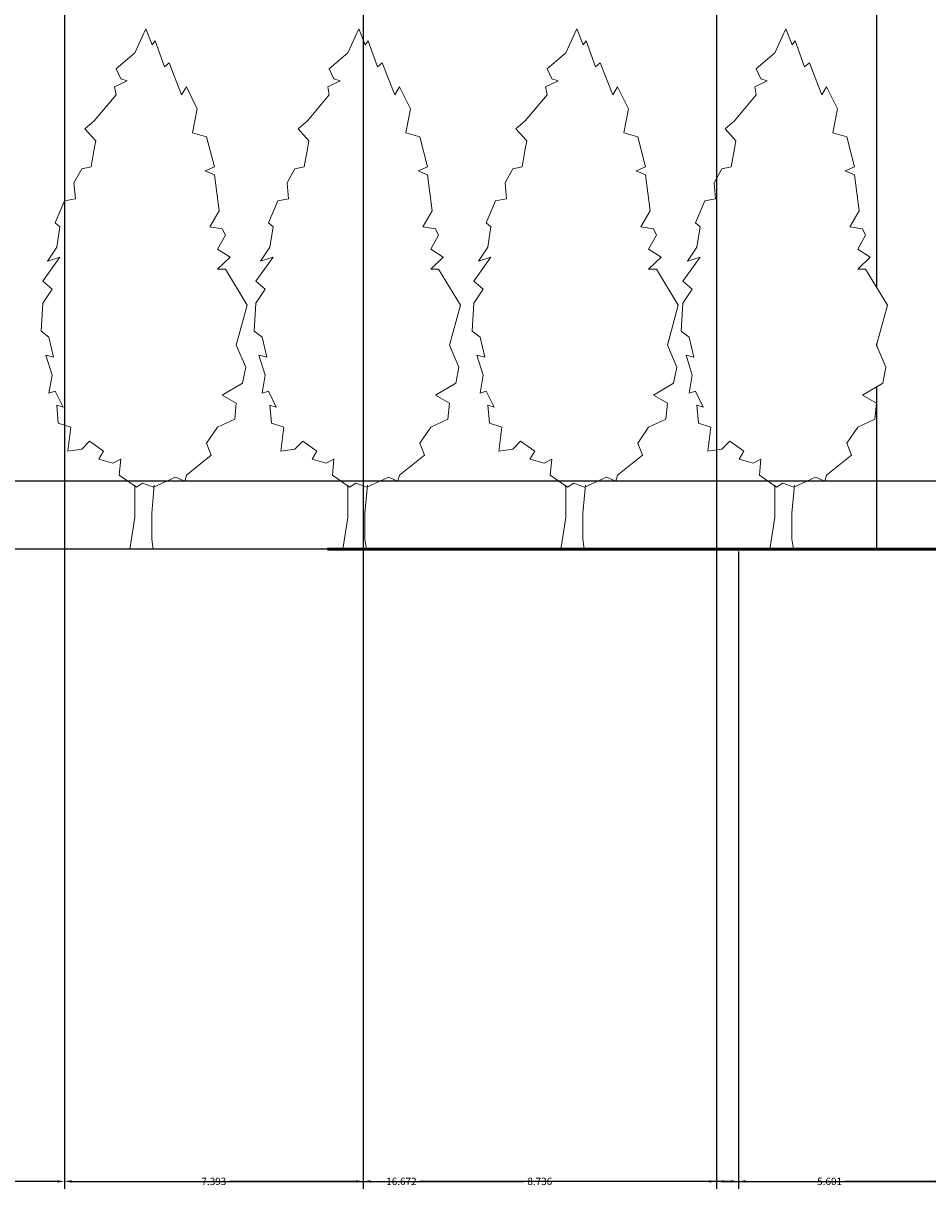
# Model space of a CAD drawing. Units: inches. Extents: x -117 to 121, y -77 to 40.
# Tile 2 of 45: x -95 to -73, y -77 to -48. Entities that reach past the tile are written whole.
import ezdxf

# ---------------------------------------------------------------- set-up
doc = ezdxf.new("R2010")
doc.units = ezdxf.units.IN
doc.header["$MEASUREMENT"] = 0
for name, color, linetype, lineweight in [('A-ANNO-DIMS', 2, 'Continuous', 18), ('A-ELEV', 7, 'Continuous', 25), ('A-ELEV-GRND', 7, 'Continuous', 50), ('L-PLNT', 3, 'Continuous', 13)]:
    doc.layers.add(name, color=color, linetype=linetype, lineweight=lineweight)
doc.styles.get("Standard").update_dxf_attribs({"font": 'arial.ttf'})
doc.dimstyles.get("Standard").update_dxf_attribs({"dimtxt": 0.18, "dimasz": 0.18, "dimexe": 0.18, "dimexo": 0.0625, "dimgap": 0.09, "dimtad": 0, "dimtih": 1, "dimtoh": 1, "dimdec": 4, "dimzin": 0, "dimdsep": 46, "dimtxsty": 'Standard', "dimcen": 0.09, "dimadec": 0, "dimazin": 0, "dimtfac": 1, "dimtdec": 4, "dimtofl": 0, "dimtmove": 0, "dimatfit": 3, "dimfxl": 1, "dimtolj": 1, "dimtzin": 0, "dimarcsym": 0})

# ---------------------------------------------------------------- blocks, each defined once
blk = doc.blocks.new('*U2')
blk.add_lwpolyline([(-2.754, 191.699), (-6.78, 182.851), (-13.682, 176.953), (-11.956, 173.266), (-9.656, 172.529), (-14.257, 170.317), (-13.682, 167.368), (-21.733, 157.783), (-25.184, 154.834), (-21.158, 150.41), (-21.733, 147.461), (-22.884, 140.825), (-26.334, 140.087), (-29.21, 134.926), (-28.635, 129.028), (-32.661, 128.291), (-36.111, 120.18), (-34.386, 118.706), (-35.536, 111.333), (-38.987, 106.171), (-34.386, 107.646), (-40.712, 98.798), (-37.261, 95.849), (-40.712, 90.688), (-41.287, 80.366), (-38.412, 78.154), (-36.686, 70.781), (-39.562, 71.518), (-37.261, 64.145), (-38.412, 57.509), (-36.111, 58.247), (-33.236, 52.348), (-35.536, 53.086), (-34.961, 46.45), (-30.36, 44.975), (-31.51, 36.128), (-26.334, 36.865), (-23.459, 39.814), (-18.283, 36.128), (-20.008, 33.178), (-14.832, 31.704), (-11.956, 33.178), (-12.531, 27.28), (-6.205, 22.856), (-3.905, 24.331), (0.121, 22.856), (8.173, 26.543), (11.624, 25.068), (12.199, 27.28), (21.4, 34.653), (19.675, 39.077), (23.701, 44.975), (30.027, 47.924), (30.602, 53.823), (25.426, 56.772), (32.903, 61.196), (34.053, 67.094), (30.602, 75.205), (34.628, 89.951), (26.576, 103.222), (23.701, 103.222), (28.302, 107.646), (23.701, 110.595), (26.576, 115.756), (25.426, 117.968), (20.825, 118.706), (24.276, 124.604), (22.551, 137.876), (19.1, 139.35), (22.551, 140.825), (19.675, 151.884), (14.499, 153.359), (16.224, 162.207), (12.199, 170.317), (10.473, 167.368), (5.872, 179.165), (4.147, 177.69), (0.696, 187.275), (-0.454, 185.8)], close=True)
for points in [[(-6.813, 23.669), (-6.813, 11.669), (-8.627, 0)], [(0.387, 23.669), (-0.576, 13.271), (-0.576, 3.686), (0, 0)]]:
    blk.add_lwpolyline(points)
blk = doc.blocks.new('*D5')
at = {"layer": 'A-ANNO-DIMS', "color": 0, "lineweight": -2, "transparency": 16777216}
for p, q in [((-94.436, -23.563), (-94.436, -77.193)), ((-106.034, -61.438), (-106.034, -77.193)), ((-105.854, -77.013), (-100.69, -77.013)), ((-94.616, -77.013), (-99.779, -77.013))]:
    blk.add_line(p, q, dxfattribs=at)
at = {"layer": 'A-ANNO-DIMS', "color": 0, "transparency": 16777216}
for points in [[(-105.854, -76.983), (-105.854, -77.043), (-106.034, -77.013)], [(-94.616, -76.983), (-94.616, -77.043), (-94.436, -77.013)]]:
    blk.add_solid(points, dxfattribs=at)
at = {"layer": 'Defpoints', "color": 0, "transparency": 16777216}
for p in [(-94.436, -23.501), (-106.034, -61.376), (-94.436, -77.013)]:
    blk.add_point(p, dxfattribs=at)
at = {"layer": 'A-ANNO-DIMS', "color": 0, "transparency": 16777216, "insert": (-100.235, -77.013), "char_height": 0.18, "attachment_point": 5}
blk.add_mtext('\\A1;11.598', dxfattribs=at)
blk = doc.blocks.new('*D6')
at = {"layer": 'A-ANNO-DIMS', "color": 0, "lineweight": -2, "transparency": 16777216}
for p, q in [((-94.436, -23.563), (-94.436, -77.193)), ((-77.763, -61.431), (-77.763, -77.193)), ((-94.256, -77.013), (-86.554, -77.013)), ((-77.943, -77.013), (-85.645, -77.013))]:
    blk.add_line(p, q, dxfattribs=at)
at = {"layer": 'A-ANNO-DIMS', "color": 0, "transparency": 16777216}
for points in [[(-94.256, -76.983), (-94.256, -77.043), (-94.436, -77.013)], [(-77.943, -76.983), (-77.943, -77.043), (-77.763, -77.013)]]:
    blk.add_solid(points, dxfattribs=at)
at = {"layer": 'Defpoints', "color": 0, "transparency": 16777216}
for p in [(-94.436, -23.501), (-77.763, -61.369), (-77.763, -77.013)]:
    blk.add_point(p, dxfattribs=at)
at = {"layer": 'A-ANNO-DIMS', "color": 0, "transparency": 16777216, "insert": (-86.099, -77.013), "char_height": 0.18, "attachment_point": 5}
blk.add_mtext('\\A1;16.672', dxfattribs=at)
blk = doc.blocks.new('*D7')
at = {"layer": 'A-ANNO-DIMS', "color": 0, "lineweight": -2, "transparency": 16777216}
for p, q in [((-77.763, -61.431), (-77.763, -77.193)), ((90.549, -61.438), (90.549, -77.193)), ((-77.583, -77.013), (6.008, -77.013)), ((90.369, -77.013), (6.778, -77.013))]:
    blk.add_line(p, q, dxfattribs=at)
at = {"layer": 'A-ANNO-DIMS', "color": 0, "transparency": 16777216}
for points in [[(-77.583, -76.983), (-77.583, -77.043), (-77.763, -77.013)], [(90.369, -76.983), (90.369, -77.043), (90.549, -77.013)]]:
    blk.add_solid(points, dxfattribs=at)
at = {"layer": 'Defpoints', "color": 0, "transparency": 16777216}
for p in [(-77.763, -61.369), (90.549, -61.376), (90.549, -77.013)]:
    blk.add_point(p, dxfattribs=at)
at = {"layer": 'A-ANNO-DIMS', "color": 0, "transparency": 16777216, "insert": (6.393, -77.013), "char_height": 0.18, "attachment_point": 5}
blk.add_mtext('\\A1;168.3', dxfattribs=at)
blk = doc.blocks.new('*D13')
at = {"layer": 'A-ANNO-DIMS', "color": 0, "lineweight": -2, "transparency": 16777216}
for p, q in [((-2.663, 27.063), (-117.024, 27.063)), ((-116.844, 26.883), (-116.844, -16.974)), ((-116.844, -61.196), (-116.844, -17.338)), ((-106.096, -61.376), (-117.024, -61.376))]:
    blk.add_line(p, q, dxfattribs=at)
at = {"layer": 'A-ANNO-DIMS', "color": 0, "transparency": 16777216}
for points in [[(-116.874, 26.883), (-116.814, 26.883), (-116.844, 27.063)], [(-116.874, -61.196), (-116.814, -61.196), (-116.844, -61.376)]]:
    blk.add_solid(points, dxfattribs=at)
at = {"layer": 'Defpoints', "color": 0, "transparency": 16777216}
for p in [(-2.6, 27.063), (-116.844, -61.376), (-106.034, -61.376)]:
    blk.add_point(p, dxfattribs=at)
at = {"layer": 'A-ANNO-DIMS', "color": 0, "transparency": 16777216, "insert": (-116.844, -17.156), "char_height": 0.18, "attachment_point": 5}
blk.add_mtext('\\A1;88.44', dxfattribs=at)
blk = doc.blocks.new('*D18')
at = {"layer": 'A-ANNO-DIMS', "color": 0, "lineweight": -2, "transparency": 16777216}
for p, q in [((-94.498, -23.501), (-117.024, -23.501)), ((-116.844, -23.681), (-116.844, -42.253)), ((-116.844, -61.189), (-116.844, -42.617)), ((-77.826, -61.369), (-117.024, -61.369))]:
    blk.add_line(p, q, dxfattribs=at)
at = {"layer": 'A-ANNO-DIMS', "color": 0, "transparency": 16777216}
for points in [[(-116.874, -23.681), (-116.814, -23.681), (-116.844, -23.501)], [(-116.874, -61.189), (-116.814, -61.189), (-116.844, -61.369)]]:
    blk.add_solid(points, dxfattribs=at)
at = {"layer": 'Defpoints', "color": 0, "transparency": 16777216}
for p in [(-94.436, -23.501), (-116.844, -61.369), (-77.763, -61.369)]:
    blk.add_point(p, dxfattribs=at)
at = {"layer": 'A-ANNO-DIMS', "color": 0, "transparency": 16777216, "insert": (-116.844, -42.435), "char_height": 0.18, "attachment_point": 5}
blk.add_mtext('\\A1;37.87', dxfattribs=at)
blk = doc.blocks.new('*D21')
at = {"layer": 'A-ANNO-DIMS', "color": 0, "lineweight": -2, "transparency": 16777216}
for p, q in [((-106.034, -61.313), (-106.034, 38.61)), ((-105.854, 38.43), (-91.382, 38.43)), ((-75.984, 38.43), (-90.455, 38.43)), ((-75.804, 8.087), (-75.804, 38.61))]:
    blk.add_line(p, q, dxfattribs=at)
at = {"layer": 'A-ANNO-DIMS', "color": 0, "transparency": 16777216}
for points in [[(-105.854, 38.46), (-105.854, 38.4), (-106.034, 38.43)], [(-75.984, 38.46), (-75.984, 38.4), (-75.804, 38.43)]]:
    blk.add_solid(points, dxfattribs=at)
at = {"layer": 'Defpoints', "color": 0, "transparency": 16777216}
for p in [(-75.804, 38.43), (-75.804, 8.025), (-106.034, -61.376)]:
    blk.add_point(p, dxfattribs=at)
at = {"layer": 'A-ANNO-DIMS', "color": 0, "transparency": 16777216, "insert": (-90.919, 38.43), "char_height": 0.18, "attachment_point": 5}
blk.add_mtext('\\A1;30.230', dxfattribs=at)
blk = doc.blocks.new('*D37')
at = {"layer": 'A-ANNO-DIMS', "color": 0, "lineweight": -2, "transparency": 16777216}
for p, q in [((-3.912, -45.613), (-117.024, -45.613)), ((-116.844, -45.793), (-116.844, -52.47)), ((-116.844, -59.512), (-116.844, -52.834)), ((-3.912, -59.692), (-117.024, -59.692))]:
    blk.add_line(p, q, dxfattribs=at)
at = {"layer": 'A-ANNO-DIMS', "color": 0, "transparency": 16777216}
for points in [[(-116.874, -45.793), (-116.814, -45.793), (-116.844, -45.613)], [(-116.874, -59.512), (-116.814, -59.512), (-116.844, -59.692)]]:
    blk.add_solid(points, dxfattribs=at)
at = {"layer": 'Defpoints', "color": 0, "transparency": 16777216}
for p in [(-116.844, -45.613), (-3.85, -45.613), (-3.85, -59.692)]:
    blk.add_point(p, dxfattribs=at)
at = {"layer": 'A-ANNO-DIMS', "color": 0, "transparency": 16777216, "insert": (-116.844, -52.652), "char_height": 0.18, "attachment_point": 5}
blk.add_mtext('\\A1;14.079', dxfattribs=at)
blk = doc.blocks.new('*D44')
at = {"layer": 'A-ANNO-DIMS', "color": 0, "lineweight": -2, "transparency": 16777216}
for p, q in [((-94.436, -23.563), (-94.436, -77.193)), ((-87.042, -23.563), (-87.042, -77.193)), ((-94.256, -77.013), (-91.132, -77.013)), ((-87.222, -77.013), (-90.346, -77.013))]:
    blk.add_line(p, q, dxfattribs=at)
at = {"layer": 'A-ANNO-DIMS', "color": 0, "transparency": 16777216}
for points in [[(-94.256, -76.983), (-94.256, -77.043), (-94.436, -77.013)], [(-87.222, -76.983), (-87.222, -77.043), (-87.042, -77.013)]]:
    blk.add_solid(points, dxfattribs=at)
at = {"layer": 'Defpoints', "color": 0, "transparency": 16777216}
for p in [(-94.436, -23.501), (-87.042, -23.501), (-87.042, -77.013)]:
    blk.add_point(p, dxfattribs=at)
at = {"layer": 'A-ANNO-DIMS', "color": 0, "transparency": 16777216, "insert": (-90.739, -77.013), "char_height": 0.18, "attachment_point": 5}
blk.add_mtext('\\A1;7.393', dxfattribs=at)
blk = doc.blocks.new('*D45')
at = {"layer": 'A-ANNO-DIMS', "color": 0, "lineweight": -2, "transparency": 16777216}
for p, q in [((-87.042, -39.778), (-87.042, -77.193)), ((-78.307, -39.778), (-78.307, -77.193)), ((-86.862, -77.013), (-83.068, -77.013)), ((-78.487, -77.013), (-82.281, -77.013))]:
    blk.add_line(p, q, dxfattribs=at)
at = {"layer": 'A-ANNO-DIMS', "color": 0, "transparency": 16777216}
for points in [[(-86.862, -76.983), (-86.862, -77.043), (-87.042, -77.013)], [(-78.487, -76.983), (-78.487, -77.043), (-78.307, -77.013)]]:
    blk.add_solid(points, dxfattribs=at)
at = {"layer": 'Defpoints', "color": 0, "transparency": 16777216}
for p in [(-87.042, -39.716), (-78.307, -39.716), (-78.307, -77.013)]:
    blk.add_point(p, dxfattribs=at)
at = {"layer": 'A-ANNO-DIMS', "color": 0, "transparency": 16777216, "insert": (-82.675, -77.013), "char_height": 0.18, "attachment_point": 5}
blk.add_mtext('\\A1;8.736', dxfattribs=at)
blk = doc.blocks.new('*D46')
at = {"layer": 'A-ANNO-DIMS', "color": 0, "lineweight": -2, "transparency": 16777216}
for p, q in [((-78.307, -39.778), (-78.307, -77.193)), ((-72.705, -39.778), (-72.705, -77.193)), ((-78.127, -77.013), (-75.882, -77.013)), ((-72.885, -77.013), (-75.13, -77.013))]:
    blk.add_line(p, q, dxfattribs=at)
at = {"layer": 'A-ANNO-DIMS', "color": 0, "transparency": 16777216}
for points in [[(-78.127, -76.983), (-78.127, -77.043), (-78.307, -77.013)], [(-72.885, -76.983), (-72.885, -77.043), (-72.705, -77.013)]]:
    blk.add_solid(points, dxfattribs=at)
at = {"layer": 'Defpoints', "color": 0, "transparency": 16777216}
for p in [(-78.307, -39.716), (-72.705, -39.716), (-72.705, -77.013)]:
    blk.add_point(p, dxfattribs=at)
at = {"layer": 'A-ANNO-DIMS', "color": 0, "transparency": 16777216, "insert": (-75.506, -77.013), "char_height": 0.18, "attachment_point": 5}
blk.add_mtext('\\A1;5.601', dxfattribs=at)

msp = doc.modelspace()

# ---------------------------------------------------------------- linework, layer by layer
at = {"layer": 'A-ELEV'}
for p, q in [((-74.3335, -54.9073), (-74.3335, -47.0788)), ((-74.3335, -56.3517), (-74.3335, -56.2811)), ((-74.3335, -61.3756), (-74.3335, -57.3495)), ((-87.9273, -61.3756), (-106.0338, -61.3756))]:
    msp.add_line(p, q, dxfattribs=at)
at = {"layer": 'A-ELEV-GRND'}
msp.add_line((90.5486, -61.3756), (-87.9273, -61.3756), dxfattribs=at)

# ---------------------------------------------------------------- block references
at = {"layer": 'L-PLNT', "xscale": 0.0671647796176818, "yscale": 0.0671647796176818, "zscale": 0.0671647796176818}
for p in [(-92.2386, -61.3752), (-86.9654, -61.3752), (-81.5737, -61.3752), (-76.4006, -61.3752)]:
    msp.add_blockref('*U2', p, dxfattribs=at)

# ---------------------------------------------------------------- dimensions: what is measured, and where the dimension line sits
at = {"layer": 'A-ANNO-DIMS'}
for base, p1, p2, override, picture, middle in [((-75.8037, 38.4297), (-106.0338, -61.3756), (-75.8037, 8.0246), {"dimdec": 3, "dimlfac": 1, "dimrnd": 0, "dimzin": 0, "dimdsep": 46, "dimlunit": 2}, '*D21', (-90.9187, 38.4297)), ((-94.4355, -77.0135), (-106.0338, -61.3756), (-94.4355, -23.5007), {"dimdec": 3, "dimlfac": 1, "dimrnd": 0, "dimzin": 0, "dimdsep": 46, "dimlunit": 2}, '*D5', (-100.2346, -77.0135)), ((-77.7631, -77.0135), (-94.4355, -23.5007), (-77.7631, -61.3689), {"dimdec": 3, "dimlfac": 1, "dimrnd": 0, "dimzin": 0, "dimdsep": 46, "dimlunit": 2}, '*D6', (-86.0993, -77.0135)), ((-87.0424, -77.0135), (-94.4355, -23.5007), (-87.0424, -23.5007), {"dimdec": 3, "dimlfac": 1, "dimrnd": 0, "dimzin": 0, "dimdsep": 46, "dimlunit": 2}, '*D44', (-90.739, -77.0135)), ((-78.3068, -77.0135), (-87.0424, -39.716), (-78.3068, -39.716), {"dimdec": 3, "dimlfac": 1, "dimrnd": 0, "dimzin": 0, "dimdsep": 46, "dimlunit": 2}, '*D45', (-82.6746, -77.0135)), ((-72.70528, -77.01347), (-78.30676, -39.71597), (-72.70528, -39.71597), {"dimdec": 3, "dimlfac": 1, "dimrnd": 0, "dimzin": 0, "dimdsep": 46, "dimlunit": 2}, '*D46', (-75.50602, -77.01347)), ((90.5486, -77.0135), (-77.7631, -61.3689), (90.5486, -61.3756), {"dimdec": 1, "dimlfac": 1, "dimrnd": 0, "dimzin": 0, "dimdsep": 46, "dimlunit": 2}, '*D7', (6.3928, -77.0135))]:
    dim = msp.add_linear_dim(base=base, p1=p1, p2=p2, dimstyle='Standard', override=override, dxfattribs=at)
    dim.commit()
    dim.dimension.update_dxf_attribs({"geometry": picture, "text_midpoint": middle})
for base, p1, p2, override, picture, middle in [((-116.8438, -61.3756), (-2.6001, 27.0634), (-106.0338, -61.3756), {"dimdec": 2, "dimlfac": 1, "dimrnd": 0, "dimzin": 0, "dimdsep": 46, "dimlunit": 2}, '*D13', (-116.8438, -17.1561)), ((-116.8438, -61.3689), (-94.4355, -23.5007), (-77.7631, -61.3689), {"dimdec": 2, "dimlfac": 1, "dimrnd": 0, "dimzin": 0, "dimdsep": 46, "dimlunit": 2}, '*D18', (-116.8438, -42.4348)), ((-116.843772, -45.612514), (-3.849514, -59.692012), (-3.849514, -45.612514), {"dimdec": 3, "dimlfac": 1, "dimrnd": 0, "dimzin": 0, "dimdsep": 46, "dimlunit": 2}, '*D37', (-116.843772, -52.652263))]:
    dim = msp.add_linear_dim(base=base, p1=p1, p2=p2, angle=90, dimstyle='Standard', override=override, dxfattribs=at)
    dim.commit()
    dim.dimension.update_dxf_attribs({"geometry": picture, "text_midpoint": middle})

doc.saveas('drawing.dxf')
